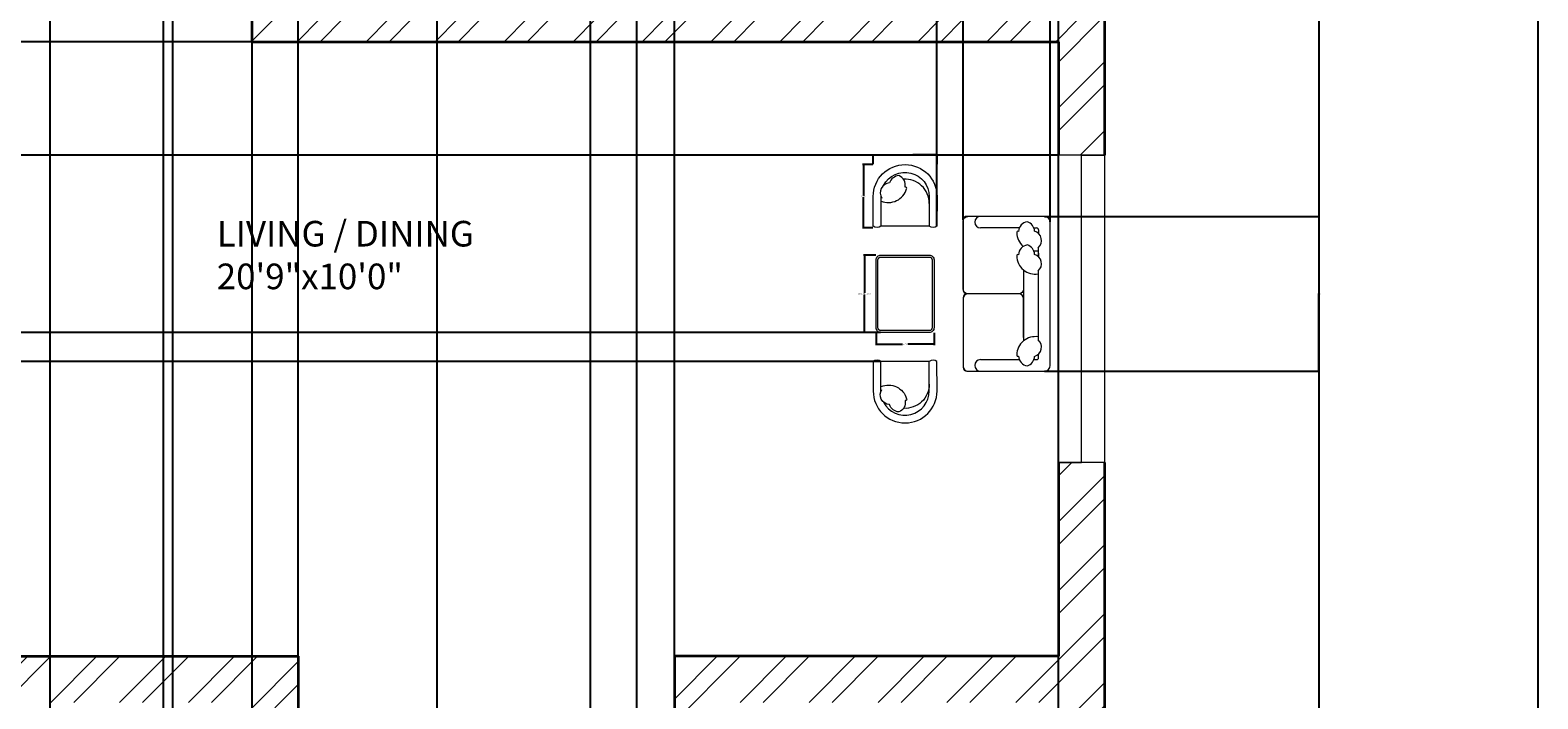
# Model space of a CAD drawing. Units: inches. Extents: x 1748 to 2382, y 1346 to 2284.
# Tile 25 of 26: x 2088 to 2382, y 1971 to 2102. Entities that reach past the tile are written whole.
import ezdxf

# ---------------------------------------------------------------- set-up
doc = ezdxf.new("R2010")
doc.units = ezdxf.units.IN
for name, color, linetype, lineweight in [('A-ANNO-DIMS', 2, 'Continuous', 18), ('A-ANNO-TTLB', 7, 'Continuous', 25), ('A-AREA-IDEN', 7, 'Continuous', 18), ('A-FURN', 8, 'Continuous', 13), ('A-GLAZ', 191, 'Continuous', 18), ('A-WALL', 7, 'Continuous', 35), ('A-WALL-PATT', 9, 'Continuous', 13)]:
    doc.layers.add(name, color=color, linetype=linetype, lineweight=lineweight)
doc.styles.get("Standard").update_dxf_attribs({"font": 'arial.ttf'})
doc.dimstyles.get("Standard").update_dxf_attribs({"dimtxt": 0.18, "dimasz": 0.18, "dimexe": 0.18, "dimexo": 0.0625, "dimgap": 0.09, "dimtad": 0, "dimtih": 1, "dimtoh": 1, "dimdec": 4, "dimzin": 0, "dimdsep": 46, "dimtxsty": 'Standard', "dimcen": 0.09, "dimadec": 0, "dimazin": 0, "dimtfac": 1, "dimtdec": 4, "dimtofl": 0, "dimtmove": 0, "dimatfit": 3, "dimfxl": 1, "dimtolj": 1, "dimtzin": 0, "dimarcsym": 0})

# ---------------------------------------------------------------- blocks, each defined once
blk = doc.blocks.new('A$C1352')
at = {"color": 0}
for points in [[(0.003, 0.053), (0.003, 0.553, -0.414214), (0.053, 0.603), (0.753, 0.603, -0.414214), (0.803, 0.553), (0.803, 0.053, -0.414214), (0.753, 0.003), (0.053, 0.003, -0.414214)], [(0.023, 0.053), (0.023, 0.553, -0.414214), (0.053, 0.583), (0.753, 0.583, -0.414214), (0.783, 0.553), (0.783, 0.053, -0.414214), (0.753, 0.023), (0.053, 0.023, -0.414214)]]:
    blk.add_lwpolyline(points, format="xyb", close=True, dxfattribs=at)
blk = doc.blocks.new('WIN-60-DEEP')
for p, q in [((0, 9), (0, 0)), ((60, 9), (0, 9)), ((60, 4.5), (60, 9)), ((60, 9), (60, 0)), ((0, 0), (0, 4.5)), ((0, 4.5), (60, 4.5)), ((0, 0), (60, 0))]:
    blk.add_line(p, q)
blk = doc.blocks.new('CHAIR-LOUNGE')
blk.add_line((1.52, 6.05), (1.51, 0.29))
at = {"ltscale": 0.03}
blk.add_lwpolyline([(1.51, 0.29, -0.369229), (0, 0.29), (0.01, 6.05, -1), (12.48, 6.04), (12.47, 0.28, -0.369229), (10.96, 0.28)], format="xyb", close=True, dxfattribs=at)
blk.add_lwpolyline([(2.05, 8.23, -0.785087), (10.96, 6.04), (10.96, 0.28)], format="xyb")
for centre, radius, start, end in [((5.21, 8.01), 2.13, 94.9999, 161.3534), ((4.35, 8.32), 1.94, 346.6403, 69.4695), ((6.24, 4.71), 4.72, 359.9461, 93.658), ((3.29, 6.8), 1.89, 92.9922, 214.1401), ((6.24, 6.05), 4.72, 178.8536, 179.9461), ((3, 8.54), 3.66, 247.0143, 344.2857), ((6.33, 7.66), 0.226, 330.6238, 113.7423)]:
    blk.add_arc(centre, radius, start, end)
blk = doc.blocks.new('*D16')
at = {"layer": 'A-ANNO-DIMS', "color": 0, "lineweight": -2, "transparency": 16777216}
for p, q in [((2252.27, 2075.42), (2252.27, 2077.41)), ((2252.45, 2077.23), (2256.99, 2077.23)), ((2264.57, 2077.23), (2260.03, 2077.23)), ((2264.75, 2075.42), (2264.75, 2077.41))]:
    blk.add_line(p, q, dxfattribs=at)
at = {"layer": 'A-ANNO-DIMS', "color": 0, "transparency": 16777216}
for points in [[(2252.45, 2077.26), (2252.45, 2077.2), (2252.27, 2077.23)], [(2264.57, 2077.26), (2264.57, 2077.2), (2264.75, 2077.23)]]:
    blk.add_solid(points, dxfattribs=at)
at = {"layer": 'Defpoints', "color": 0, "transparency": 16777216}
for p in [(2264.75, 2077.23), (2252.27, 2075.36), (2264.75, 2075.36)]:
    blk.add_point(p, dxfattribs=at)
at = {"layer": 'A-ANNO-DIMS', "color": 0, "transparency": 16777216, "insert": (2258.51, 2077.23), "char_height": 0.18, "attachment_point": 5}
blk.add_mtext('\\A1;LOUNGE CHAIR 12 TYP.', dxfattribs=at)
blk = doc.blocks.new('*D17')
at = {"layer": 'A-ANNO-DIMS', "color": 0, "lineweight": -2, "transparency": 16777216}
for p, q in [((2252.21, 2075.36), (2250.22, 2075.36)), ((2250.4, 2075.18), (2250.4, 2069.35)), ((2250.4, 2063.16), (2250.4, 2068.99)), ((2252.21, 2062.98), (2250.22, 2062.98))]:
    blk.add_line(p, q, dxfattribs=at)
at = {"layer": 'A-ANNO-DIMS', "color": 0, "transparency": 16777216}
for points in [[(2250.37, 2075.18), (2250.43, 2075.18), (2250.4, 2075.36)], [(2250.37, 2063.16), (2250.43, 2063.16), (2250.4, 2062.98)]]:
    blk.add_solid(points, dxfattribs=at)
at = {"layer": 'Defpoints', "color": 0, "transparency": 16777216}
for p in [(2250.4, 2075.36), (2252.27, 2075.36), (2252.27, 2062.98)]:
    blk.add_point(p, dxfattribs=at)
at = {"layer": 'A-ANNO-DIMS', "color": 0, "transparency": 16777216, "insert": (2250.4, 2069.17), "char_height": 0.18, "attachment_point": 5}
blk.add_mtext('\\A1;12 TYP.', dxfattribs=at)
blk = doc.blocks.new('*D24')
at = {"layer": 'A-ANNO-DIMS', "color": 0, "lineweight": -2, "transparency": 16777216}
for p, q in [((2252.77, 2057.69), (2250.39, 2057.69)), ((2250.57, 2057.51), (2250.57, 2050.31)), ((2250.57, 2042.75), (2250.57, 2049.95)), ((2252.77, 2042.57), (2250.39, 2042.57))]:
    blk.add_line(p, q, dxfattribs=at)
at = {"layer": 'A-ANNO-DIMS', "color": 0, "transparency": 16777216}
for points in [[(2250.54, 2057.51), (2250.6, 2057.51), (2250.57, 2057.69)], [(2250.54, 2042.75), (2250.6, 2042.75), (2250.57, 2042.57)]]:
    blk.add_solid(points, dxfattribs=at)
at = {"layer": 'Defpoints', "color": 0, "transparency": 16777216}
for p in [(2252.84, 2057.69), (2250.57, 2042.57), (2252.84, 2042.57)]:
    blk.add_point(p, dxfattribs=at)
at = {"layer": 'A-ANNO-DIMS', "color": 0, "transparency": 16777216, "insert": (2250.57, 2050.13), "char_height": 0.18, "attachment_point": 5}
blk.add_mtext('\\A1;COFFEE TABLE 15 TYP.', dxfattribs=at)
blk = doc.blocks.new('*D25')
at = {"layer": 'A-ANNO-DIMS', "color": 0, "lineweight": -2, "transparency": 16777216}
for p, q in [((2252.84, 2042.51), (2252.84, 2040.13)), ((2264.17, 2042.51), (2264.17, 2040.13)), ((2253.02, 2040.31), (2257.99, 2040.31)), ((2263.99, 2040.31), (2259.02, 2040.31))]:
    blk.add_line(p, q, dxfattribs=at)
at = {"layer": 'A-ANNO-DIMS', "color": 0, "transparency": 16777216}
for points in [[(2253.02, 2040.34), (2253.02, 2040.28), (2252.84, 2040.31)], [(2263.99, 2040.34), (2263.99, 2040.28), (2264.17, 2040.31)]]:
    blk.add_solid(points, dxfattribs=at)
at = {"layer": 'Defpoints', "color": 0, "transparency": 16777216}
for p in [(2252.84, 2042.57), (2264.17, 2042.57), (2264.17, 2040.31)]:
    blk.add_point(p, dxfattribs=at)
at = {"layer": 'A-ANNO-DIMS', "color": 0, "transparency": 16777216, "insert": (2258.5, 2040.31), "char_height": 0.18, "attachment_point": 5}
blk.add_mtext('\\A1;11 TYP.', dxfattribs=at)
blk = doc.blocks.new('*D35')
at = {"layer": 'A-ANNO-DIMS', "color": 0, "lineweight": -2, "transparency": 16777216}
for p, q in [((2297.52, 2232.85), (2339.54, 2232.85)), ((2339.36, 2232.67), (2339.36, 1850.53)), ((2339.36, 1468.03), (2339.36, 1850.17)), ((2297.52, 1467.85), (2339.54, 1467.85))]:
    blk.add_line(p, q, dxfattribs=at)
at = {"layer": 'A-ANNO-DIMS', "color": 0, "transparency": 16777216}
for points in [[(2339.33, 2232.67), (2339.39, 2232.67), (2339.36, 2232.85)], [(2339.33, 1468.03), (2339.39, 1468.03), (2339.36, 1467.85)]]:
    blk.add_solid(points, dxfattribs=at)
at = {"layer": 'Defpoints', "color": 0, "transparency": 16777216}
for p in [(2297.46, 2232.85), (2339.36, 2232.85), (2297.46, 1467.85)]:
    blk.add_point(p, dxfattribs=at)
at = {"layer": 'A-ANNO-DIMS', "color": 0, "transparency": 16777216, "insert": (2339.36, 1850.35), "char_height": 0.18, "attachment_point": 5}
blk.add_mtext('\\A1;765', dxfattribs=at)
blk = doc.blocks.new('*D38')
at = {"layer": 'A-ANNO-DIMS', "color": 0, "lineweight": -2, "transparency": 16777216}
for p, q in [((2113.63, 1859.41), (2113.63, 2274.93)), ((2113.81, 2274.75), (2121.84, 2274.75)), ((2130.78, 2274.75), (2122.75, 2274.75)), ((2130.96, 1859.41), (2130.96, 2274.93))]:
    blk.add_line(p, q, dxfattribs=at)
at = {"layer": 'A-ANNO-DIMS', "color": 0, "transparency": 16777216}
for points in [[(2113.81, 2274.78), (2113.81, 2274.72), (2113.63, 2274.75)], [(2130.78, 2274.78), (2130.78, 2274.72), (2130.96, 2274.75)]]:
    blk.add_solid(points, dxfattribs=at)
at = {"layer": 'Defpoints', "color": 0, "transparency": 16777216}
for p in [(2130.96, 2274.75), (2113.63, 1859.35), (2130.96, 1859.35)]:
    blk.add_point(p, dxfattribs=at)
at = {"layer": 'A-ANNO-DIMS', "color": 0, "transparency": 16777216, "insert": (2122.29, 2274.75), "char_height": 0.18, "attachment_point": 5}
blk.add_mtext('\\A1;17.334', dxfattribs=at)
blk = doc.blocks.new('*D39')
at = {"layer": 'A-ANNO-DIMS', "color": 0, "lineweight": -2, "transparency": 16777216}
for p, q in [((2139.96, 1734.91), (2139.96, 2274.93)), ((2140.14, 2274.75), (2168.14, 2274.75)), ((2196.89, 2274.75), (2168.89, 2274.75)), ((2197.07, 1734.91), (2197.07, 2274.93))]:
    blk.add_line(p, q, dxfattribs=at)
at = {"layer": 'A-ANNO-DIMS', "color": 0, "transparency": 16777216}
for points in [[(2140.14, 2274.78), (2140.14, 2274.72), (2139.96, 2274.75)], [(2196.89, 2274.78), (2196.89, 2274.72), (2197.07, 2274.75)]]:
    blk.add_solid(points, dxfattribs=at)
at = {"layer": 'Defpoints', "color": 0, "transparency": 16777216}
for p in [(2197.07, 2274.75), (2139.96, 1734.85), (2197.07, 1734.85)]:
    blk.add_point(p, dxfattribs=at)
at = {"layer": 'A-ANNO-DIMS', "color": 0, "transparency": 16777216, "insert": (2168.52, 2274.75), "char_height": 0.18, "attachment_point": 5}
blk.add_mtext('\\A1;57.11', dxfattribs=at)
blk = doc.blocks.new('*D40')
at = {"layer": 'A-ANNO-DIMS', "color": 0, "lineweight": -2, "transparency": 16777216}
for p, q in [((2206.07, 1734.91), (2206.07, 2274.93)), ((2206.25, 2274.75), (2246.87, 2274.75)), ((2288.28, 2274.75), (2247.66, 2274.75)), ((2288.46, 1734.91), (2288.46, 2274.93))]:
    blk.add_line(p, q, dxfattribs=at)
at = {"layer": 'A-ANNO-DIMS', "color": 0, "transparency": 16777216}
for points in [[(2206.25, 2274.78), (2206.25, 2274.72), (2206.07, 2274.75)], [(2288.28, 2274.78), (2288.28, 2274.72), (2288.46, 2274.75)]]:
    blk.add_solid(points, dxfattribs=at)
at = {"layer": 'Defpoints', "color": 0, "transparency": 16777216}
for p in [(2288.46, 2274.75), (2206.07, 1734.85), (2288.46, 1734.85)]:
    blk.add_point(p, dxfattribs=at)
at = {"layer": 'A-ANNO-DIMS', "color": 0, "transparency": 16777216, "insert": (2247.27, 2274.75), "char_height": 0.18, "attachment_point": 5}
blk.add_mtext('\\A1;82.39', dxfattribs=at)
blk = doc.blocks.new('*D52')
at = {"layer": 'A-ANNO-DIMS', "color": 0, "lineweight": -2, "transparency": 16777216}
for p, q in [((2064.07, 2223.79), (2064.07, 1360.47)), ((2091.4, 2223.79), (2091.4, 1360.47)), ((2064.25, 1360.65), (2077.34, 1360.65)), ((2091.22, 1360.65), (2078.13, 1360.65))]:
    blk.add_line(p, q, dxfattribs=at)
at = {"layer": 'A-ANNO-DIMS', "color": 0, "transparency": 16777216}
for points in [[(2064.25, 1360.68), (2064.25, 1360.62), (2064.07, 1360.65)], [(2091.22, 1360.68), (2091.22, 1360.62), (2091.4, 1360.65)]]:
    blk.add_solid(points, dxfattribs=at)
at = {"layer": 'Defpoints', "color": 0, "transparency": 16777216}
for p in [(2064.07, 2223.85), (2091.4, 2223.85), (2091.4, 1360.65)]:
    blk.add_point(p, dxfattribs=at)
at = {"layer": 'A-ANNO-DIMS', "color": 0, "transparency": 16777216, "insert": (2077.73, 1360.65), "char_height": 0.18, "attachment_point": 5}
blk.add_mtext('\\A1;27.33', dxfattribs=at)
blk = doc.blocks.new('*D53')
at = {"layer": 'A-ANNO-DIMS', "color": 0, "lineweight": -2, "transparency": 16777216}
for p, q in [((2115.4, 2223.79), (2115.4, 1360.47)), ((2167.02, 2223.79), (2167.02, 1360.47)), ((2115.58, 1360.65), (2140.81, 1360.65)), ((2166.84, 1360.65), (2141.6, 1360.65))]:
    blk.add_line(p, q, dxfattribs=at)
at = {"layer": 'A-ANNO-DIMS', "color": 0, "transparency": 16777216}
for points in [[(2115.58, 1360.68), (2115.58, 1360.62), (2115.4, 1360.65)], [(2166.84, 1360.68), (2166.84, 1360.62), (2167.02, 1360.65)]]:
    blk.add_solid(points, dxfattribs=at)
at = {"layer": 'Defpoints', "color": 0, "transparency": 16777216}
for p in [(2115.4, 2223.85), (2167.02, 2223.85), (2167.02, 1360.65)]:
    blk.add_point(p, dxfattribs=at)
at = {"layer": 'A-ANNO-DIMS', "color": 0, "transparency": 16777216, "insert": (2141.21, 1360.65), "char_height": 0.18, "attachment_point": 5}
blk.add_mtext('\\A1;51.62', dxfattribs=at)
blk = doc.blocks.new('*D57')
at = {"layer": 'A-ANNO-DIMS', "color": 0, "lineweight": -2, "transparency": 16777216}
for p, q in [((2288.4, 2099.35), (1779.88, 2099.35)), ((1780.06, 2099.17), (1780.06, 2088.46)), ((1780.06, 2077.38), (1780.06, 2088.09)), ((2288.4, 2077.2), (1779.88, 2077.2))]:
    blk.add_line(p, q, dxfattribs=at)
at = {"layer": 'A-ANNO-DIMS', "color": 0, "transparency": 16777216}
for points in [[(1780.03, 2099.17), (1780.09, 2099.17), (1780.06, 2099.35)], [(1780.03, 2077.38), (1780.09, 2077.38), (1780.06, 2077.2)]]:
    blk.add_solid(points, dxfattribs=at)
at = {"layer": 'Defpoints', "color": 0, "transparency": 16777216}
for p in [(1780.06, 2099.35), (2288.46, 2099.35), (2288.46, 2077.2)]:
    blk.add_point(p, dxfattribs=at)
at = {"layer": 'A-ANNO-DIMS', "color": 0, "transparency": 16777216, "insert": (1780.06, 2088.28), "char_height": 0.18, "attachment_point": 5}
blk.add_mtext('\\A1;22.15', dxfattribs=at)
blk = doc.blocks.new('*D58')
at = {"layer": 'A-ANNO-DIMS', "color": 0, "lineweight": -2, "transparency": 16777216}
for p, q in [((2269.84, 2064.55), (2269.84, 2274.93)), ((2270.02, 2274.75), (2277.89, 2274.75)), ((2286.67, 2274.75), (2278.8, 2274.75)), ((2286.85, 2064.18), (2286.85, 2274.93))]:
    blk.add_line(p, q, dxfattribs=at)
at = {"layer": 'A-ANNO-DIMS', "color": 0, "transparency": 16777216}
for points in [[(2270.02, 2274.78), (2270.02, 2274.72), (2269.84, 2274.75)], [(2286.67, 2274.78), (2286.67, 2274.72), (2286.85, 2274.75)]]:
    blk.add_solid(points, dxfattribs=at)
at = {"layer": 'Defpoints', "color": 0, "transparency": 16777216}
for p in [(2286.85, 2274.75), (2269.84, 2064.49), (2286.85, 2064.11)]:
    blk.add_point(p, dxfattribs=at)
at = {"layer": 'A-ANNO-DIMS', "color": 0, "transparency": 16777216, "insert": (2278.34, 2274.75), "char_height": 0.18, "attachment_point": 5}
blk.add_mtext('\\A1;17.006', dxfattribs=at)
blk = doc.blocks.new('*D59')
at = {"layer": 'A-ANNO-DIMS', "color": 0, "lineweight": -2, "transparency": 16777216}
for p, q in [((2285.78, 2065.25), (2339.54, 2065.25)), ((2339.36, 2065.07), (2339.36, 2050.31)), ((2339.36, 2035.19), (2339.36, 2049.95)), ((2285.78, 2035.01), (2339.54, 2035.01))]:
    blk.add_line(p, q, dxfattribs=at)
at = {"layer": 'A-ANNO-DIMS', "color": 0, "transparency": 16777216}
for points in [[(2339.33, 2065.07), (2339.39, 2065.07), (2339.36, 2065.25)], [(2339.33, 2035.19), (2339.39, 2035.19), (2339.36, 2035.01)]]:
    blk.add_solid(points, dxfattribs=at)
at = {"layer": 'Defpoints', "color": 0, "transparency": 16777216}
for p in [(2285.71, 2065.25), (2339.36, 2065.25), (2285.71, 2035.01)]:
    blk.add_point(p, dxfattribs=at)
at = {"layer": 'A-ANNO-DIMS', "color": 0, "transparency": 16777216, "insert": (2339.36, 2050.13), "char_height": 0.18, "attachment_point": 5}
blk.add_mtext('\\A1;30.23', dxfattribs=at)
blk = doc.blocks.new('*D62')
at = {"layer": 'A-ANNO-DIMS', "color": 0, "lineweight": -2, "transparency": 16777216}
for p, q in [((2264.74, 2063.41), (2264.74, 2274.93)), ((2264.92, 2274.75), (2266.9, 2274.75)), ((2269.66, 2274.75), (2267.68, 2274.75)), ((2269.84, 2064.55), (2269.84, 2274.93))]:
    blk.add_line(p, q, dxfattribs=at)
at = {"layer": 'A-ANNO-DIMS', "color": 0, "transparency": 16777216}
for points in [[(2264.92, 2274.78), (2264.92, 2274.72), (2264.74, 2274.75)], [(2269.66, 2274.78), (2269.66, 2274.72), (2269.84, 2274.75)]]:
    blk.add_solid(points, dxfattribs=at)
at = {"layer": 'Defpoints', "color": 0, "transparency": 16777216}
for p in [(2269.84, 2274.75), (2264.74, 2063.35), (2269.84, 2064.49)]:
    blk.add_point(p, dxfattribs=at)
at = {"layer": 'A-ANNO-DIMS', "color": 0, "transparency": 16777216, "insert": (2267.29, 2274.75), "char_height": 0.18, "attachment_point": 5}
blk.add_mtext('\\A1;5.102', dxfattribs=at)
blk = doc.blocks.new('*D63')
at = {"layer": 'A-ANNO-DIMS', "color": 0, "lineweight": -2, "transparency": 16777216}
for p, q in [((2253.72, 2042.57), (1779.88, 2042.57)), ((1780.06, 2042.39), (1780.06, 2039.92)), ((1780.06, 2037.08), (1780.06, 2039.55)), ((2253.72, 2036.9), (1779.88, 2036.9))]:
    blk.add_line(p, q, dxfattribs=at)
at = {"layer": 'A-ANNO-DIMS', "color": 0, "transparency": 16777216}
for points in [[(1780.03, 2042.39), (1780.09, 2042.39), (1780.06, 2042.57)], [(1780.03, 2037.08), (1780.09, 2037.08), (1780.06, 2036.9)]]:
    blk.add_solid(points, dxfattribs=at)
at = {"layer": 'Defpoints', "color": 0, "transparency": 16777216}
for p in [(1780.06, 2042.57), (2253.78, 2042.57), (2253.78, 2036.9)]:
    blk.add_point(p, dxfattribs=at)
at = {"layer": 'A-ANNO-DIMS', "color": 0, "transparency": 16777216, "insert": (1780.06, 2039.74), "char_height": 0.18, "attachment_point": 5}
blk.add_mtext('\\A1;5.673', dxfattribs=at)
blk = doc.blocks.new('*D73')
at = {"layer": 'A-ANNO-DIMS', "color": 0, "lineweight": -2, "transparency": 16777216}
for p, q in [((2139.96, 1979.41), (2139.96, 2274.93)), ((2140.14, 2274.75), (2176.39, 2274.75)), ((2213.28, 2274.75), (2177.03, 2274.75)), ((2213.46, 1979.41), (2213.46, 2274.93))]:
    blk.add_line(p, q, dxfattribs=at)
at = {"layer": 'A-ANNO-DIMS', "color": 0, "transparency": 16777216}
for points in [[(2140.14, 2274.78), (2140.14, 2274.72), (2139.96, 2274.75)], [(2213.28, 2274.78), (2213.28, 2274.72), (2213.46, 2274.75)]]:
    blk.add_solid(points, dxfattribs=at)
at = {"layer": 'Defpoints', "color": 0, "transparency": 16777216}
for p in [(2213.46, 2274.75), (2139.96, 1979.35), (2213.46, 1979.35)]:
    blk.add_point(p, dxfattribs=at)
at = {"layer": 'A-ANNO-DIMS', "color": 0, "transparency": 16777216, "insert": (2176.71, 2274.75), "char_height": 0.18, "attachment_point": 5}
blk.add_mtext('\\A1;73.5', dxfattribs=at)

msp = doc.modelspace()

# ---------------------------------------------------------------- hatches: boundary and pattern name
at = {"layer": 'A-WALL-PATT'}
h = msp.add_hatch(dxfattribs=at)
h.set_pattern_fill('ANSI32', color=256)
h.paths.add_polyline_path([(1908.4445, 2232.8497), (1821.9607, 2232.8497), (1821.9607, 2223.8497), (1865.4607, 2223.8497), (1865.4607, 2209.9185), (1869.9607, 2209.9185), (1869.9607, 2223.8497), (1908.4445, 2223.8497), (1908.4445, 2228.3497)])
h.paths.add_polyline_path([(2040.0683, 2232.8497), (1968.4445, 2232.8497), (1968.4445, 2223.8497), (2025.9607, 2223.8497), (2025.9607, 2130.3497), (2032.1341, 2130.3497), (2032.1341, 2132.5997), (2032.1341, 2134.8497), (2030.4607, 2134.8497), (2030.4607, 2223.8497), (2040.0683, 2223.8497)])
h.paths.add_polyline_path([(2091.3969, 2232.8497), (2064.0683, 2232.8497), (2064.0683, 2223.8497), (2078.4607, 2223.8497), (2078.4607, 2134.8497), (2051.1563, 2134.8497), (2051.1563, 2130.3497), (2078.4607, 2130.3497), (2078.4607, 2128.6813), (2082.9607, 2128.6813), (2082.9607, 2130.3497), (2086.1879, 2130.3497), (2086.1879, 2132.5997), (2086.1879, 2134.8497), (2082.9607, 2134.8497), (2082.9607, 2223.8497), (2091.3969, 2223.8497), (2091.3969, 2228.3497)])
h.paths.add_polyline_path([(2167.0164, 2232.8497), (2115.3969, 2232.8497), (2115.3969, 2223.8497), (2130.9607, 2223.8497), (2130.9607, 2134.8497), (2106.9607, 2134.8497), (2106.9607, 2130.3497), (2135.4607, 2130.3497), (2135.4607, 2223.8497), (2167.0164, 2223.8497), (2167.0164, 2228.3497)])
h.paths.add_polyline_path([(1869.9607, 2149.9185), (1865.4607, 2149.9185), (1865.4607, 2127.8942), (1869.9607, 2127.8942)])
h.paths.add_polyline_path([(2082.9607, 2104.4871), (2080.7107, 2104.4871), (2078.4607, 2104.4871), (2078.4607, 2103.8497), (1869.9607, 2103.8497), (1869.9607, 2108.6062), (1867.7107, 2108.6062), (1865.4607, 2108.6062), (1865.4607, 2103.8497), (1821.9607, 2103.8497), (1821.9607, 2099.3497), (1865.4607, 2099.3497), (1865.4607, 2094.7509), (1869.9607, 2094.7509), (1869.9607, 2099.3497), (2025.9607, 2099.3497), (2025.9607, 2096.4326), (2030.4607, 2096.4326), (2030.4607, 2099.3497), (2082.9607, 2099.3497)])
h.paths.add_polyline_path([(1928.9457, 1401.1212), (2176.8693, 1401.1212), (2176.8693, 1438.214), (1928.9457, 1438.214)], flags=9)
h.paths.add_polyline_path([(2122.2668, 2048.1927), (2177.9387, 2048.1927), (2177.9387, 2066.85), (2122.2668, 2066.85)], flags=9)
h.paths.add_polyline_path([(2272.688, 2153.8197), (2272.688, 2216.746), (2262.3845, 2216.746), (2262.3845, 2153.8197)], flags=9)
h.paths.add_polyline_path([(2157.2928, 2166.5593), (2196.3822, 2166.5593), (2196.3822, 2185.2167), (2157.2928, 2185.2167)], flags=9)
h.paths.add_polyline_path([(2089.3407, 2162.0698), (2124.3987, 2162.0698), (2124.3987, 2180.7272), (2089.3407, 2180.7272)], flags=9)
h.paths.add_polyline_path([(2037.4521, 2160.0913), (2072.5101, 2160.0913), (2072.5101, 2178.7486), (2037.4521, 2178.7486)], flags=9)
h.paths.add_polyline_path([(1884.7894, 2104.1554), (1923.6297, 2104.1554), (1923.6297, 2122.8127), (1884.7894, 2122.8127)], flags=9)
h.paths.add_polyline_path([(1851.2832, 2142.9749), (1851.2832, 2199.3051), (1840.9796, 2199.3051), (1840.9796, 2142.9749)], flags=9)
h.paths.add_polyline_path([(1844.8763, 2017.2834), (1844.8763, 2073.6136), (1834.5728, 2073.6136), (1834.5728, 2017.2834)], flags=9)
h.paths.add_polyline_path([(1897.1577, 2073.1279), (1935.9981, 2073.1279), (1935.9981, 2091.7853), (1897.1577, 2091.7853)], flags=9)
h.paths.add_polyline_path([(1952.3395, 1802.4231), (2008.0114, 1802.4231), (2008.0114, 1821.0805), (1952.3395, 1821.0805)], flags=9)
h.paths.add_polyline_path([(1978.8184, 1857.6841), (2017.7338, 1857.6841), (2017.7338, 1876.3415), (1978.8184, 1876.3415)], flags=9)
h.paths.add_polyline_path([(1979.6513, 1925.9516), (2008.8089, 1925.9516), (2008.8089, 1944.6089), (1979.6513, 1944.6089)], flags=9)
h.paths.add_polyline_path([(1838.5553, 1860.3527), (1877.3957, 1860.3527), (1877.3957, 1879.01), (1838.5553, 1879.01)], flags=9)
h.paths.add_polyline_path([(1883.9018, 1787.3013), (1883.9018, 1843.6315), (1873.5983, 1843.6315), (1873.5983, 1787.3013)], flags=9)
h.paths.add_polyline_path([(1873.7079, 1509.1938), (1873.7079, 1583.7709), (1863.4044, 1583.7709), (1863.4044, 1509.1938)], flags=9)
h.paths.add_polyline_path([(1916.2259, 1603.3681), (1955.0663, 1603.3681), (1955.0663, 1622.0254), (1916.2259, 1622.0254)], flags=9)
h.paths.add_polyline_path([(1876.3013, 1636.757), (1876.3013, 1693.0871), (1865.9978, 1693.0871), (1865.9978, 1636.757)], flags=9)
h.paths.add_polyline_path([(1921.3138, 1521.8316), (1964.0662, 1521.8316), (1964.0662, 1540.489), (1921.3138, 1540.489)], flags=9)
h.paths.add_polyline_path([(2017.5657, 1497.5078), (2046.7983, 1497.5078), (2046.7983, 1516.1651), (2017.5657, 1516.1651)], flags=9)
h.paths.add_polyline_path([(2066.8661, 1499.3902), (2096.0988, 1499.3902), (2096.0988, 1518.0475), (2066.8661, 1518.0475)], flags=9)
h.paths.add_polyline_path([(2155.4835, 1571.6596), (2198.2358, 1571.6596), (2198.2358, 1590.3169), (2155.4835, 1590.3169)], flags=9)
h.paths.add_polyline_path([(2094.9136, 1664.6812), (2150.5855, 1664.6812), (2150.5855, 1683.3386), (2094.9136, 1683.3386)], flags=9)
h.paths.add_polyline_path([(2257.6902, 1863.1628), (2269.8935, 1863.1628), (2269.8935, 1873.4664), (2257.6902, 1873.4664)], flags=9)
h.paths.add_polyline_path([(2164.0748, 1880.3089), (2189.8694, 1880.3089), (2189.8694, 1890.6124), (2164.0748, 1890.6124)], flags=9)
h.paths.add_polyline_path([(2239.4394, 1931.0585), (2268.8187, 1931.0585), (2268.8187, 1949.7159), (2239.4394, 1949.7159)], flags=9)
h = msp.add_hatch(dxfattribs=at)
h.set_pattern_fill('ANSI32', color=256)
h.paths.add_polyline_path([(2297.4607, 2232.8497), (2203.0164, 2232.8497), (2203.0164, 2223.8497), (2244.9607, 2223.8497), (2244.9607, 2127.8554), (2249.4607, 2127.8554), (2249.4607, 2223.8497), (2297.4607, 2223.8497)])
h.paths.add_polyline_path([(2297.4607, 2103.8497), (2249.4607, 2103.8497), (2249.4607, 2106.7497), (2247.2107, 2106.7497), (2244.9607, 2106.7497), (2244.9607, 2103.8497), (2130.9607, 2103.8497), (2130.9607, 2099.3497), (2288.4607, 2099.3497), (2288.4607, 2077.2008), (2297.4607, 2077.2008)])
h.paths.add_polyline_path([(1928.9457, 1401.1212), (2176.8693, 1401.1212), (2176.8693, 1438.214), (1928.9457, 1438.214)], flags=9)
h.paths.add_polyline_path([(2122.2668, 2048.1927), (2177.9387, 2048.1927), (2177.9387, 2066.85), (2122.2668, 2066.85)], flags=9)
h.paths.add_polyline_path([(2272.688, 2153.8197), (2272.688, 2216.746), (2262.3845, 2216.746), (2262.3845, 2153.8197)], flags=25)
h.paths.add_polyline_path([(2157.2928, 2166.5593), (2196.3822, 2166.5593), (2196.3822, 2185.2167), (2157.2928, 2185.2167)], flags=9)
h.paths.add_polyline_path([(2089.3407, 2162.0698), (2124.3987, 2162.0698), (2124.3987, 2180.7272), (2089.3407, 2180.7272)], flags=9)
h.paths.add_polyline_path([(2037.4521, 2160.0913), (2072.5101, 2160.0913), (2072.5101, 2178.7486), (2037.4521, 2178.7486)], flags=9)
h.paths.add_polyline_path([(1884.7894, 2104.1554), (1923.6297, 2104.1554), (1923.6297, 2122.8127), (1884.7894, 2122.8127)], flags=9)
h.paths.add_polyline_path([(1851.2832, 2142.9749), (1851.2832, 2199.3051), (1840.9796, 2199.3051), (1840.9796, 2142.9749)], flags=9)
h.paths.add_polyline_path([(1844.8763, 2017.2834), (1844.8763, 2073.6136), (1834.5728, 2073.6136), (1834.5728, 2017.2834)], flags=9)
h.paths.add_polyline_path([(1897.1577, 2073.1279), (1935.9981, 2073.1279), (1935.9981, 2091.7853), (1897.1577, 2091.7853)], flags=9)
h.paths.add_polyline_path([(1952.3395, 1802.4231), (2008.0114, 1802.4231), (2008.0114, 1821.0805), (1952.3395, 1821.0805)], flags=9)
h.paths.add_polyline_path([(1978.8184, 1857.6841), (2017.7338, 1857.6841), (2017.7338, 1876.3415), (1978.8184, 1876.3415)], flags=9)
h.paths.add_polyline_path([(1979.6513, 1925.9516), (2008.8089, 1925.9516), (2008.8089, 1944.6089), (1979.6513, 1944.6089)], flags=9)
h.paths.add_polyline_path([(1838.5553, 1860.3527), (1877.3957, 1860.3527), (1877.3957, 1879.01), (1838.5553, 1879.01)], flags=9)
h.paths.add_polyline_path([(1883.9018, 1787.3013), (1883.9018, 1843.6315), (1873.5983, 1843.6315), (1873.5983, 1787.3013)], flags=9)
h.paths.add_polyline_path([(1873.7079, 1509.1938), (1873.7079, 1583.7709), (1863.4044, 1583.7709), (1863.4044, 1509.1938)], flags=9)
h.paths.add_polyline_path([(1916.2259, 1603.3681), (1955.0663, 1603.3681), (1955.0663, 1622.0254), (1916.2259, 1622.0254)], flags=9)
h.paths.add_polyline_path([(1876.3013, 1636.757), (1876.3013, 1693.0871), (1865.9978, 1693.0871), (1865.9978, 1636.757)], flags=9)
h.paths.add_polyline_path([(1921.3138, 1521.8316), (1964.0662, 1521.8316), (1964.0662, 1540.489), (1921.3138, 1540.489)], flags=9)
h.paths.add_polyline_path([(2017.5657, 1497.5078), (2046.7983, 1497.5078), (2046.7983, 1516.1651), (2017.5657, 1516.1651)], flags=9)
h.paths.add_polyline_path([(2066.8661, 1499.3902), (2096.0988, 1499.3902), (2096.0988, 1518.0475), (2066.8661, 1518.0475)], flags=9)
h.paths.add_polyline_path([(2155.4835, 1571.6596), (2198.2358, 1571.6596), (2198.2358, 1590.3169), (2155.4835, 1590.3169)], flags=9)
h.paths.add_polyline_path([(2094.9136, 1664.6812), (2150.5855, 1664.6812), (2150.5855, 1683.3386), (2094.9136, 1683.3386)], flags=9)
h.paths.add_polyline_path([(2257.6902, 1863.1628), (2269.8935, 1863.1628), (2269.8935, 1873.4664), (2257.6902, 1873.4664)], flags=9)
h.paths.add_polyline_path([(2164.0748, 1880.3089), (2189.8694, 1880.3089), (2189.8694, 1890.6124), (2164.0748, 1890.6124)], flags=9)
h.paths.add_polyline_path([(2239.4394, 1931.0585), (2268.8187, 1931.0585), (2268.8187, 1949.7159), (2239.4394, 1949.7159)], flags=9)
h = msp.add_hatch(dxfattribs=at)
h.set_pattern_fill('ANSI32', color=256)
h.paths.add_polyline_path([(1919.6777, 1476.8497), (1900.6426, 1476.8497), (1900.6426, 1522.0826), (1898.3926, 1522.0826), (1896.1426, 1522.0826), (1896.1426, 1476.8497), (1857.1426, 1476.8497), (1857.1426, 1467.8497), (1896.1426, 1467.8497), (1919.6777, 1467.8497), (1919.6777, 1472.3497)])
h.paths.add_polyline_path([(2018.7873, 1472.3497), (2018.7873, 1476.8497), (2010.9607, 1476.8497), (2010.9607, 1560.8497), (2034.9607, 1560.8497), (2034.9607, 1565.3497), (2006.4607, 1565.3497), (2006.4607, 1476.8497), (1955.6777, 1476.8497), (1955.6777, 1467.8497), (2018.7873, 1467.8497)])
h.paths.add_polyline_path([(2152.3354, 1472.3497), (2152.3354, 1476.8497), (2115.9607, 1476.8497), (2115.9607, 1565.3497), (2109.2204, 1565.3497), (2109.2204, 1563.0997), (2109.2204, 1560.8497), (2111.4607, 1560.8497), (2111.4607, 1476.8497), (2095.3617, 1476.8497), (2095.3617, 1467.8497), (2152.3354, 1467.8497)])
h.paths.add_polyline_path([(2071.3617, 1476.8497), (2063.4607, 1476.8497), (2063.4607, 1560.8497), (2090.1865, 1560.8497), (2090.1865, 1565.3497), (2063.4607, 1565.3497), (2063.4607, 1572.5485), (2061.2107, 1572.5485), (2058.9607, 1572.5485), (2058.9607, 1565.3497), (2055.6281, 1565.3497), (2055.6281, 1560.8497), (2058.9607, 1560.8497), (2058.9607, 1476.8497), (2042.7873, 1476.8497), (2042.7873, 1467.8497), (2071.3617, 1467.8497), (2071.3617, 1472.3497)])
h.paths.add_polyline_path([(2297.4607, 1506.5652), (2288.4607, 1506.5652), (2288.4607, 1476.8497), (2212.3354, 1476.8497), (2212.3354, 1467.8497), (2297.4607, 1467.8497)])
h.paths.add_polyline_path([(2297.4607, 1645.3038), (2288.4607, 1645.3038), (2288.4607, 1605.8497), (2058.9607, 1605.8497), (2058.9607, 1600.1857), (2061.2107, 1600.1857), (2063.4607, 1600.1857), (2063.4607, 1601.3497), (2288.4607, 1601.3497), (2288.4607, 1566.5652), (2297.4607, 1566.5652)])
h.paths.add_polyline_path([(2010.9607, 1609.0561), (2008.7107, 1609.0561), (2006.4607, 1609.0561), (2006.4607, 1605.8497), (1900.6426, 1605.8497), (1900.6426, 1609.7171), (1898.3926, 1609.7171), (1896.1426, 1609.7171), (1896.1426, 1605.8497), (1857.1426, 1605.8497), (1857.1426, 1601.3497), (1896.1426, 1601.3497), (1896.1426, 1542.5447), (1900.6426, 1542.5447), (1900.6426, 1601.3497), (2010.9607, 1601.3497)])
h.paths.add_polyline_path([(1928.9457, 1401.1212), (2176.8693, 1401.1212), (2176.8693, 1438.214), (1928.9457, 1438.214)], flags=9)
h.paths.add_polyline_path([(2122.2668, 2048.1927), (2177.9387, 2048.1927), (2177.9387, 2066.85), (2122.2668, 2066.85)], flags=9)
h.paths.add_polyline_path([(2272.688, 2153.8197), (2272.688, 2216.746), (2262.3845, 2216.746), (2262.3845, 2153.8197)], flags=9)
h.paths.add_polyline_path([(2157.2928, 2166.5593), (2196.3822, 2166.5593), (2196.3822, 2185.2167), (2157.2928, 2185.2167)], flags=9)
h.paths.add_polyline_path([(2089.3407, 2162.0698), (2124.3987, 2162.0698), (2124.3987, 2180.7272), (2089.3407, 2180.7272)], flags=9)
h.paths.add_polyline_path([(2037.4521, 2160.0913), (2072.5101, 2160.0913), (2072.5101, 2178.7486), (2037.4521, 2178.7486)], flags=9)
h.paths.add_polyline_path([(1884.7894, 2104.1554), (1923.6297, 2104.1554), (1923.6297, 2122.8127), (1884.7894, 2122.8127)], flags=9)
h.paths.add_polyline_path([(1851.2832, 2142.9749), (1851.2832, 2199.3051), (1840.9796, 2199.3051), (1840.9796, 2142.9749)], flags=9)
h.paths.add_polyline_path([(1844.8763, 2017.2834), (1844.8763, 2073.6136), (1834.5728, 2073.6136), (1834.5728, 2017.2834)], flags=9)
h.paths.add_polyline_path([(1897.1577, 2073.1279), (1935.9981, 2073.1279), (1935.9981, 2091.7853), (1897.1577, 2091.7853)], flags=9)
h.paths.add_polyline_path([(1952.3395, 1802.4231), (2008.0114, 1802.4231), (2008.0114, 1821.0805), (1952.3395, 1821.0805)], flags=9)
h.paths.add_polyline_path([(1978.8184, 1857.6841), (2017.7338, 1857.6841), (2017.7338, 1876.3415), (1978.8184, 1876.3415)], flags=9)
h.paths.add_polyline_path([(1979.6513, 1925.9516), (2008.8089, 1925.9516), (2008.8089, 1944.6089), (1979.6513, 1944.6089)], flags=9)
h.paths.add_polyline_path([(1838.5553, 1860.3527), (1877.3957, 1860.3527), (1877.3957, 1879.01), (1838.5553, 1879.01)], flags=9)
h.paths.add_polyline_path([(1883.9018, 1787.3013), (1883.9018, 1843.6315), (1873.5983, 1843.6315), (1873.5983, 1787.3013)], flags=9)
h.paths.add_polyline_path([(1873.7079, 1509.1938), (1873.7079, 1583.7709), (1863.4044, 1583.7709), (1863.4044, 1509.1938)], flags=9)
h.paths.add_polyline_path([(1916.2259, 1603.3681), (1955.0663, 1603.3681), (1955.0663, 1622.0254), (1916.2259, 1622.0254)], flags=9)
h.paths.add_polyline_path([(1876.3013, 1636.757), (1876.3013, 1693.0871), (1865.9978, 1693.0871), (1865.9978, 1636.757)], flags=9)
h.paths.add_polyline_path([(1921.3138, 1521.8316), (1964.0662, 1521.8316), (1964.0662, 1540.489), (1921.3138, 1540.489)], flags=9)
h.paths.add_polyline_path([(2017.5657, 1497.5078), (2046.7983, 1497.5078), (2046.7983, 1516.1651), (2017.5657, 1516.1651)], flags=9)
h.paths.add_polyline_path([(2066.8661, 1499.3902), (2096.0988, 1499.3902), (2096.0988, 1518.0475), (2066.8661, 1518.0475)], flags=9)
h.paths.add_polyline_path([(2155.4835, 1571.6596), (2198.2358, 1571.6596), (2198.2358, 1590.3169), (2155.4835, 1590.3169)], flags=25)
h.paths.add_polyline_path([(2094.9136, 1664.6812), (2150.5855, 1664.6812), (2150.5855, 1683.3386), (2094.9136, 1683.3386)], flags=9)
h.paths.add_polyline_path([(2257.6902, 1863.1628), (2269.8935, 1863.1628), (2269.8935, 1873.4664), (2257.6902, 1873.4664)], flags=9)
h.paths.add_polyline_path([(2164.0748, 1880.3089), (2189.8694, 1880.3089), (2189.8694, 1890.6124), (2164.0748, 1890.6124)], flags=9)
h.paths.add_polyline_path([(2239.4394, 1931.0585), (2268.8187, 1931.0585), (2268.8187, 1949.7159), (2239.4394, 1949.7159)], flags=9)
h = msp.add_hatch(dxfattribs=at)
h.set_pattern_fill('ANSI32', color=256)
h.paths.add_polyline_path([(1900.6426, 1652.723), (1896.1426, 1652.723), (1896.1426, 1629.9029), (1900.6426, 1629.9029)])
h.paths.add_polyline_path([(2206.0699, 1859.3497), (2197.0699, 1859.3497), (2197.0699, 1734.8497), (2206.0699, 1734.8497)], flags=17)
h.paths.add_polyline_path([(2297.4607, 1865.3269), (2288.4607, 1865.3269), (2288.4607, 1734.8497), (2206.0699, 1734.8497), (2180.4551, 1734.8497), (2180.4551, 1725.8497), (2197.0699, 1725.8497), (2206.0699, 1725.8497), (2288.4607, 1725.8497), (2288.4607, 1705.3038), (2297.4607, 1705.3038)])
h.paths.add_polyline_path([(2139.9607, 1815.8001), (2135.4607, 1815.8001), (2130.9607, 1815.8001), (2130.9607, 1734.8497), (1900.6426, 1734.8497), (1900.6426, 1738.9477), (1898.3926, 1738.9477), (1896.1426, 1738.9477), (1896.1426, 1734.8497), (1857.1426, 1734.8497), (1857.1426, 1725.8497), (1896.1426, 1725.8497), (1896.1426, 1712.723), (1900.6426, 1712.723), (1900.6426, 1725.8497), (2006.4607, 1725.8497), (2006.4607, 1637.448), (2010.9607, 1637.448), (2010.9607, 1725.8497), (2139.9607, 1725.8497), (2147.389, 1725.8497), (2147.389, 1730.3497), (2147.389, 1734.8497), (2139.9607, 1734.8497)])
h.paths.add_polyline_path([(2149.8497, 1917.8497), (2149.8497, 1922.3497), (2139.9607, 1922.3497), (2139.9607, 1979.3497), (2030.4607, 1979.3497), (2030.4607, 2069.8971), (2028.2107, 2069.8971), (2025.9607, 2069.8971), (2025.9607, 1979.3497), (1869.9607, 1979.3497), (1869.9607, 1998.93), (1865.4607, 1998.93), (1865.4607, 1979.3497), (1821.9607, 1979.3497), (1821.9607, 1952.7922), (1826.9306, 1952.7922), (1830.9607, 1952.7922), (1830.9607, 1970.3497), (1962.9607, 1970.3497), (1962.9607, 1926.5713), (1967.4607, 1926.5713), (1967.4607, 1970.3497), (2027.4607, 1970.3497), (2027.4607, 1898.3497), (2004.9604, 1898.3497), (2004.9604, 1893.8497), (2027.4607, 1893.8497), (2027.4607, 1859.3497), (1958.8973, 1859.3497), (1958.8973, 1854.8497), (2047.917, 1854.8497), (2047.917, 1859.3497), (2031.9607, 1859.3497), (2031.9607, 1970.3497), (2130.9607, 1970.3497), (2130.9607, 1859.3497), (2104.9565, 1859.3497), (2104.9565, 1854.8497), (2130.9607, 1854.8497), (2130.9607, 1849.0684), (2139.9607, 1849.0684), (2139.9607, 1913.3497), (2149.8497, 1913.3497)])
h.paths.add_polyline_path([(1928.9996, 1859.3497), (1830.9607, 1859.3497), (1830.9607, 1892.7922), (1821.9607, 1892.7922), (1821.9607, 1854.8497), (1896.1426, 1854.8497), (1896.1426, 1836.6443), (1898.378, 1836.6443), (1900.6426, 1836.6443), (1900.6426, 1854.8497), (1928.9996, 1854.8497), (1928.9996, 1857.0997)])
h.paths.add_polyline_path([(1980.9604, 1896.0997), (1980.9604, 1898.3497), (1967.4607, 1898.3497), (1967.4607, 1902.3846), (1962.9607, 1902.3846), (1962.9607, 1859.3497), (1967.4607, 1859.3497), (1967.4607, 1893.8497), (1980.9604, 1893.8497)], flags=17)
h.paths.add_polyline_path([(1900.6426, 1776.6443), (1896.1426, 1776.6443), (1896.1426, 1758.0891), (1900.6426, 1758.0891)], flags=17)
h.paths.add_polyline_path([(2297.4607, 2017.2008), (2288.4607, 2017.2008), (2288.4607, 1979.3497), (2213.4607, 1979.3497), (2213.4607, 1922.3497), (2183.3516, 1922.3497), (2183.3516, 1913.3497), (2213.4607, 1913.3497), (2236.234, 1913.3497), (2236.234, 1922.3497), (2222.4607, 1922.3497), (2222.4607, 1931.3497), (2222.4607, 1970.3497), (2288.4607, 1970.3497), (2288.4607, 1922.3497), (2272.1921, 1922.3497), (2272.1921, 1913.3497), (2288.4607, 1913.3497), (2288.4607, 1901.3269), (2297.4607, 1901.3269)])

# ---------------------------------------------------------------- linework, layer by layer
at = {"layer": 'A-ANNO-TTLB'}
msp.add_lwpolyline([(1747.8112, 2284.3704), (2382.1361, 2284.3704), (2382.1361, 1346.4899), (1747.8112, 1346.4899)], close=True, dxfattribs=at)
at = {"layer": 'A-FURN'}
for p, q in [((2280.8079, 2062.98), (2273.2431, 2062.98)), ((2283.6762, 2062.98), (2284.2024, 2062.98)), ((2284.5803, 2062.602), (2284.5803, 2061.9068)), ((2284.5803, 2057.3703), (2284.5803, 2059.1787)), ((2284.5803, 2058.0655), (2284.5803, 2057.3703)), ((2284.5803, 2041.0836), (2284.5803, 2054.6421)), ((2273.2431, 2037.2824), (2280.8079, 2037.2824)), ((2283.6762, 2037.2824), (2284.2024, 2037.2824)), ((2284.5803, 2037.6603), (2284.5803, 2038.3555))]:
    msp.add_line(p, q, dxfattribs=at)
at = {"layer": 'A-FURN', "ltscale": 0.03}
msp.add_lwpolyline([(2270.5977, 2050.1219, 0.41421356), (2269.8419, 2049.3661), (2269.8419, 2035.7707, 0.41421356), (2270.5977, 2035.0149), (2285.714, 2035.0149, 0.41421356), (2286.8477, 2036.1486), (2286.8477, 2064.1137, 0.41421356), (2285.714, 2065.2474), (2270.5977, 2065.2474, 0.41421356), (2269.8419, 2064.4916), (2269.8419, 2050.8963, 0.41421356), (2270.5977, 2050.1404)], format="xyb", dxfattribs=at)
at = {"layer": 'A-FURN'}
for points in [[(2281.6515, 2054.7937), (2281.6515, 2051.0759, -0.41421356), (2280.7067, 2050.1312), (2270.7867, 2050.1312, -0.41421356), (2269.8419, 2051.0759), (2269.8419, 2064.3026, -0.41421356), (2270.7867, 2065.2474)], [(2281.6515, 2041.5754), (2281.6515, 2049.1864, 0.41421356), (2280.7067, 2050.1312), (2270.7867, 2050.1312, 0.41421356), (2269.8419, 2049.1864), (2269.8419, 2035.9597, 0.41421356), (2270.7867, 2035.0149)]]:
    msp.add_lwpolyline(points, format="xyb", dxfattribs=at)
msp.add_lwpolyline([(2281.6515, 2054.7937), (2281.6515, 2040.932)], dxfattribs=at)
for centre, radius, start, end in [((2273.2431, 2064.1137), 1.1337, 90, 180), ((2273.2431, 2064.1137), 1.1337, 180, 270), ((2280.534, 2062.1143), 0.226, 52.154994, 195.27353), ((2283.9725, 2062.1577), 3.658, 181.611631, 229.375991), ((2282.6143, 2062.2677), 1.9418, 96.427858, 179.256998), ((2281.6995, 2062.1835), 2.1311, 4.543938, 70.89739), ((2283.2674, 2060.5427), 1.8933, 311.757236, 72.905096), ((2284.2024, 2062.602), 0.3779, 0, 90), ((2284.2024, 2062.602), 0.3779, 0, 90), ((2282.6143, 2057.7311), 1.9418, 96.427858, 179.256998), ((2281.6995, 2057.647), 2.1311, 4.543938, 70.89739), ((2280.534, 2057.5778), 0.226, 52.154994, 195.27353), ((2283.9725, 2057.6211), 3.658, 181.611631, 278.88305), ((2283.9725, 2062.1577), 3.658, 264.880983, 278.88305), ((2283.2674, 2056.0062), 1.8933, 311.757236, 72.905096), ((2283.9725, 2038.1046), 3.658, 81.11695, 178.388369), ((2283.2674, 2039.7196), 1.8933, 287.094904, 48.242764), ((2273.2431, 2036.1486), 1.1337, 90, 180), ((2273.2431, 2036.1486), 1.1337, 180, 270), ((2280.534, 2038.148), 0.226, 164.72647, 307.845006), ((2282.6143, 2037.9946), 1.9418, 180.743002, 263.572142), ((2281.6995, 2038.0788), 2.1311, 289.10261, 355.456062), ((2284.2024, 2037.6603), 0.3779, 270, 0)]:
    msp.add_arc(centre, radius, start, end, dxfattribs=at)
at = {"layer": 'A-WALL'}
for p, q in [((2297.4607, 2232.8497), (2297.4607, 2077.2008)), ((2130.9607, 2099.3497), (2130.9607, 2103.8497)), ((2130.9607, 2099.3497), (2288.4607, 2099.3497)), ((2288.4607, 2099.3497), (2288.4607, 2077.2008)), ((2288.4607, 2017.2008), (2288.4607, 1979.3497)), ((2297.4607, 2017.2008), (2297.4607, 1901.3269)), ((2030.4607, 1979.3497), (2139.9607, 1979.3497)), ((2139.9607, 1979.3497), (2139.9607, 1922.3497)), ((2288.4607, 1979.3497), (2213.4607, 1979.3497)), ((2213.4607, 1979.3497), (2213.4607, 1922.3497))]:
    msp.add_line(p, q, dxfattribs=at)

# ---------------------------------------------------------------- block references
at = {"layer": 'A-FURN'}
msp.add_blockref('CHAIR-LOUNGE', (2252.269, 2063.074), dxfattribs=at)
at = {"layer": 'A-FURN', "ltscale": 0.03, "xscale": 18.89529246734385, "yscale": 18.89529246734385, "zscale": 18.89529246734385, "rotation": 270}
msp.add_blockref('A$C1352', (2252.7796, 2057.74), dxfattribs=at)
at = {"layer": 'A-FURN', "extrusion": (0, 0, -1), "zscale": -1, "rotation": 180}
msp.add_blockref('CHAIR-LOUNGE', (-2252.269, 2037.1883), dxfattribs=at)
at = {"layer": 'A-GLAZ', "extrusion": (0, 0, -1), "zscale": -1, "rotation": 90.00000000000003}
msp.add_blockref('WIN-60-DEEP', (-2288.461, 2017.2004), dxfattribs=at)

# ---------------------------------------------------------------- texts
at = {"layer": 'A-AREA-IDEN', "insert": (2124.0284, 2064.362), "char_height": 5, "attachment_point": 1}
msp.add_mtext_dynamic_manual_height_columns('LIVING / DINING\\P20\'9"x10\'0"', width=281.556752, gutter_width=12.5, heights=[0], dxfattribs=at)

# ---------------------------------------------------------------- dimensions: what is measured, and where the dimension line sits
at = {"layer": 'A-ANNO-DIMS'}
for base, p1, p2, override, picture, middle in [((2130.9607, 2274.7497), (2113.6268, 1859.3497), (2130.9607, 1859.3497), {"dimdec": 3, "dimlfac": 1, "dimrnd": 0, "dimzin": 0, "dimdsep": 46, "dimlunit": 2}, '*D38', (2122.2937, 2274.7497)), ((2197.0699, 2274.7497), (2139.9607, 1734.8497), (2197.0699, 1734.8497), {"dimdec": 2, "dimlfac": 1, "dimrnd": 0, "dimzin": 0, "dimdsep": 46, "dimlunit": 2}, '*D39', (2168.5153, 2274.7497)), ((2213.4607, 2274.7497), (2139.9607, 1979.3497), (2213.4607, 1979.3497), {"dimdec": 1, "dimlfac": 1, "dimrnd": 0, "dimzin": 0, "dimdsep": 46, "dimlunit": 2}, '*D73', (2176.7107, 2274.7497)), ((2288.4607, 2274.7497), (2206.0699, 1734.8497), (2288.4607, 1734.8497), {"dimdec": 2, "dimlfac": 1, "dimrnd": 0, "dimzin": 0, "dimdsep": 46, "dimlunit": 2}, '*D40', (2247.2653, 2274.7497)), ((2269.8419, 2274.7497), (2264.7402, 2063.352), (2269.8419, 2064.4916), {"dimdec": 3, "dimlfac": 1, "dimrnd": 0, "dimzin": 0, "dimdsep": 46, "dimlunit": 2}, '*D62', (2267.2911, 2274.7497)), ((2286.8477, 2274.7497), (2269.8419, 2064.4916), (2286.8477, 2064.1137), {"dimdec": 3, "dimlfac": 1, "dimrnd": 0, "dimzin": 0, "dimdsep": 46, "dimlunit": 2}, '*D58', (2278.3448, 2274.7497)), ((2091.3969, 1360.6451), (2064.0683, 2223.8497), (2091.3969, 2223.8497), {"dimdec": 2, "dimlfac": 1, "dimrnd": 0, "dimzin": 0, "dimdsep": 46, "dimlunit": 2}, '*D52', (2077.7326, 1360.6451)), ((2167.0164, 1360.6451), (2115.3969, 2223.8497), (2167.0164, 2223.8497), {"dimdec": 2, "dimlfac": 1, "dimrnd": 0, "dimzin": 0, "dimdsep": 46, "dimlunit": 2}, '*D53', (2141.2066, 1360.6451))]:
    dim = msp.add_linear_dim(base=base, p1=p1, p2=p2, dimstyle='Standard', override=override, dxfattribs=at)
    dim.commit()
    dim.dimension.update_dxf_attribs({"geometry": picture, "text_midpoint": middle})
for base, p1, p2, override, picture, middle in [((2339.3607, 2232.8497), (2297.4607, 1467.8497), (2297.4607, 2232.8497), {"dimdec": 0, "dimlfac": 1, "dimrnd": 0, "dimzin": 0, "dimdsep": 46, "dimlunit": 2}, '*D35', (2339.3607, 1850.3497)), ((1780.0607, 2099.3497), (2288.4607, 2077.2008), (2288.4607, 2099.3497), {"dimdec": 2, "dimlfac": 1, "dimrnd": 0, "dimzin": 0, "dimdsep": 46, "dimlunit": 2}, '*D57', (1780.0607, 2088.2752)), ((2339.3607, 2065.2474), (2285.714, 2035.0149), (2285.714, 2065.2474), {"dimdec": 2, "dimlfac": 1, "dimrnd": 0, "dimzin": 0, "dimdsep": 46, "dimlunit": 2}, '*D59', (2339.3607, 2050.1312)), ((1780.0607, 2042.573), (2253.7809, 2036.9), (2253.7809, 2042.573), {"dimdec": 3, "dimlfac": 1, "dimrnd": 0, "dimzin": 0, "dimdsep": 46, "dimlunit": 2}, '*D63', (1780.0607, 2039.7365))]:
    dim = msp.add_linear_dim(base=base, p1=p1, p2=p2, angle=90, dimstyle='Standard', override=override, dxfattribs=at)
    dim.commit()
    dim.dimension.update_dxf_attribs({"geometry": picture, "text_midpoint": middle})
for base, p1, p2, text, picture, middle in [((2264.7489, 2077.2331), (2252.2693, 2075.3612), (2264.7489, 2075.3612), 'LOUNGE CHAIR <> TYP.', '*D16', (2258.5091, 2077.2331)), ((2264.1733, 2040.3056), (2252.8362, 2042.573), (2264.1733, 2042.573), '<> TYP.', '*D25', (2258.5048, 2040.3056))]:
    dim = msp.add_linear_dim(base=base, p1=p1, p2=p2, text=text, dimstyle='Standard', override={"dimdec": 0, "dimlfac": 1, "dimrnd": 0, "dimzin": 0, "dimdsep": 46, "dimlunit": 2}, dxfattribs=at)
    dim.commit()
    dim.dimension.update_dxf_attribs({"geometry": picture, "text_midpoint": middle})
for base, p1, p2, angle, text, picture, middle in [((2250.3974, 2075.3612), (2252.2693, 2062.9803), (2252.2693, 2075.3612), 90, '<> TYP.', '*D17', (2250.3974, 2069.1707)), ((2250.5687, 2042.573), (2252.8362, 2057.6893), (2252.8362, 2042.573), 270, 'COFFEE TABLE <> TYP.', '*D24', (2250.5687, 2050.1312))]:
    dim = msp.add_linear_dim(base=base, p1=p1, p2=p2, angle=angle, text=text, dimstyle='Standard', override={"dimdec": 0, "dimlfac": 1, "dimrnd": 0, "dimzin": 0, "dimdsep": 46, "dimlunit": 2}, dxfattribs=at)
    dim.commit()
    dim.dimension.update_dxf_attribs({"geometry": picture, "text_midpoint": middle})

doc.saveas('drawing.dxf')
